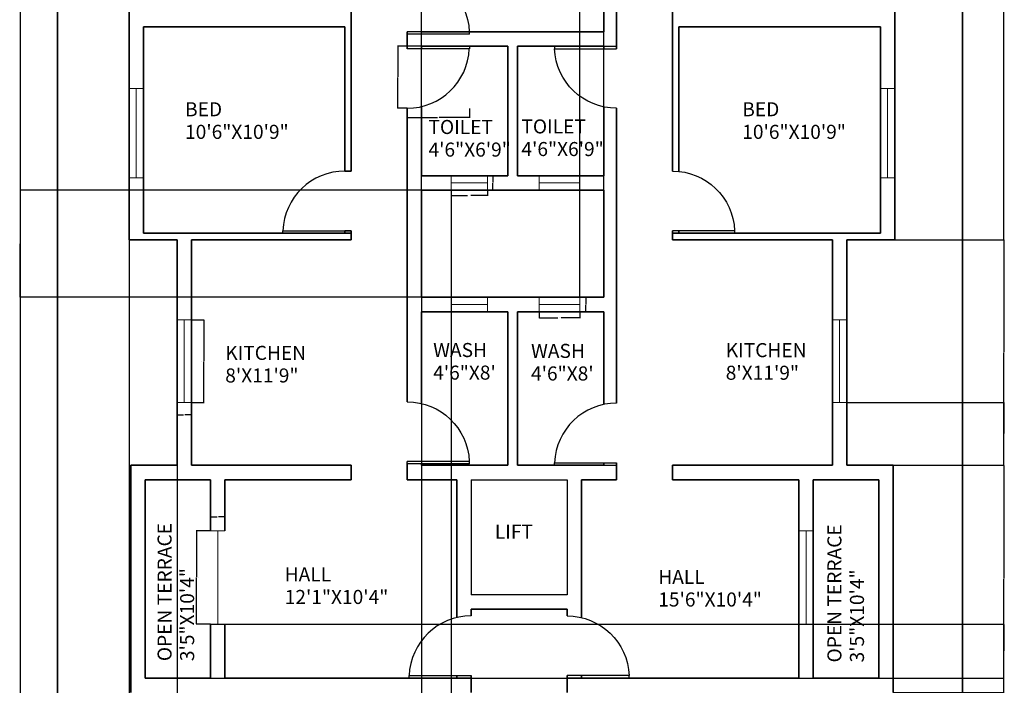
# Model space of a CAD drawing. Units: feet. Extents: x 100807 to 101423, y 154875 to 156331.
# Tile 2 of 8: x 100807 to 101423, y 155624 to 156040. Entities that reach past the tile are written whole.
import ezdxf

# ---------------------------------------------------------------- set-up
doc = ezdxf.new("R2010")
doc.units = ezdxf.units.FT
for name, color, linetype, lineweight in [('A-ANNO-DIMS', 2, 'Continuous', 18), ('A-ANNO-TTLB', 7, 'Continuous', 35), ('A-AREA-IDEN', 7, 'Continuous', 25), ('A-DOOR', 4, 'Continuous', 25), ('A-EQPM-ELEV', 8, 'Continuous', 25), ('A-GLAZ', 4, 'Continuous', 18), ('A-WALL', 7, 'Continuous', 35)]:
    doc.layers.add(name, color=color, linetype=linetype, lineweight=lineweight)
doc.styles.get("Standard").update_dxf_attribs({"font": 'arial.ttf'})
doc.dimstyles.get("Standard").update_dxf_attribs({"dimtxt": 0.18, "dimasz": 0.18, "dimexe": 0.18, "dimexo": 0.0625, "dimgap": 0.09, "dimtad": 0, "dimtih": 1, "dimtoh": 1, "dimdec": 4, "dimzin": 0, "dimdsep": 46, "dimtxsty": 'Standard', "dimcen": 0.09, "dimadec": 0, "dimazin": 0, "dimtfac": 1, "dimtdec": 4, "dimtofl": 0, "dimtmove": 0, "dimatfit": 3, "dimfxl": 1, "dimtolj": 1, "dimtzin": 0, "dimarcsym": 0})

# ---------------------------------------------------------------- blocks, each defined once
blk = doc.blocks.new('DR-36')
for p, q in [((0, 36), (0, 0)), ((0, 36), (1.5, 36)), ((1.5, 36), (1.5, 0)), ((0, 0), (1.5, 0))]:
    blk.add_line(p, q)
blk.add_arc((0, 0), 36, 0, 87.6141)
blk = doc.blocks.new('VENT-COURT-A')
for p, q in [((0, 9), (0, 0)), ((22.83, 9), (22.83, 0)), ((22.83, 4.5), (0, 4.5))]:
    blk.add_line(p, q)
blk = doc.blocks.new('VENT-COURT-B')
for p, q in [((0, 9), (0, 0)), ((25.42, 9), (25.42, 0)), ((25.42, 4.5), (0, 4.5))]:
    blk.add_line(p, q)
blk = doc.blocks.new('WIN-KITCHEN')
for p, q in [((0, 51.58), (9, 51.58)), ((4.5, 51.58), (4.5, 0)), ((0, 0), (9, 0))]:
    blk.add_line(p, q)
blk = doc.blocks.new('WIN-BED-SIDE')
for p, q in [((0, 55.85), (9, 55.85)), ((4.5, 55.85), (4.5, 0)), ((0, 0), (9, 0))]:
    blk.add_line(p, q)
blk = doc.blocks.new('WIN-TERRACE')
for p, q in [((0, 58.29), (9, 58.29)), ((4.5, 58.29), (4.5, 0)), ((0, 0), (9, 0))]:
    blk.add_line(p, q)
blk = doc.blocks.new('LIFT-OUTLINE')
for p, q in [((0, 72), (0, 0)), ((0, 72), (60, 72)), ((60, 72), (60, 0)), ((60, 72), (60, 0)), ((60, 0), (0, 0))]:
    blk.add_line(p, q)
blk = doc.blocks.new('*D12')
at = {"layer": 'A-ANNO-DIMS', "color": 0, "lineweight": -2, "transparency": 16777216}
for p, q in [((101049.09, 156023.58), (101043.15, 156023.58)), ((101043.33, 156023.4), (101043.33, 156004.33)), ((101043.33, 155984.89), (101043.33, 156003.96)), ((101049.09, 155984.71), (101043.15, 155984.71))]:
    blk.add_line(p, q, dxfattribs=at)
at = {"layer": 'A-ANNO-DIMS', "color": 0, "transparency": 16777216}
for points in [[(101043.3, 156023.4), (101043.36, 156023.4), (101043.33, 156023.58)], [(101043.3, 155984.89), (101043.36, 155984.89), (101043.33, 155984.71)]]:
    blk.add_solid(points, dxfattribs=at)
at = {"layer": 'Defpoints', "color": 0, "transparency": 16777216}
for p in [(101049.16, 156023.58), (101043.33, 155984.71), (101049.16, 155984.71)]:
    blk.add_point(p, dxfattribs=at)
at = {"layer": 'A-ANNO-DIMS', "color": 0, "transparency": 16777216, "insert": (101043.33, 156004.14), "char_height": 0.18, "attachment_point": 5}
blk.add_mtext('\\A1;DOOR 39 TYP.', dxfattribs=at)
blk = doc.blocks.new('*D13')
at = {"layer": 'A-ANNO-DIMS', "color": 0, "lineweight": -2, "transparency": 16777216}
for p, q in [((101049.16, 155984.65), (101049.16, 155978.7)), ((101088.02, 155984.65), (101088.02, 155978.7)), ((101049.34, 155978.88), (101068.06, 155978.88)), ((101087.84, 155978.88), (101069.12, 155978.88))]:
    blk.add_line(p, q, dxfattribs=at)
at = {"layer": 'A-ANNO-DIMS', "color": 0, "transparency": 16777216}
for points in [[(101049.34, 155978.91), (101049.34, 155978.85), (101049.16, 155978.88)], [(101087.84, 155978.91), (101087.84, 155978.85), (101088.02, 155978.88)]]:
    blk.add_solid(points, dxfattribs=at)
at = {"layer": 'Defpoints', "color": 0, "transparency": 16777216}
for p in [(101049.16, 155984.71), (101088.02, 155984.71), (101088.02, 155978.88)]:
    blk.add_point(p, dxfattribs=at)
at = {"layer": 'A-ANNO-DIMS', "color": 0, "transparency": 16777216, "insert": (101068.59, 155978.88), "char_height": 0.18, "attachment_point": 5}
blk.add_mtext('\\A1;39 TYP.', dxfattribs=at)
blk = doc.blocks.new('*D14')
at = {"layer": 'A-ANNO-DIMS', "color": 0, "lineweight": -2, "transparency": 16777216}
for p, q in [((101076.57, 155933.52), (101076.57, 155929.97)), ((101099.4, 155933.52), (101099.4, 155929.97)), ((101076.75, 155930.15), (101086.96, 155930.15)), ((101099.22, 155930.15), (101089, 155930.15))]:
    blk.add_line(p, q, dxfattribs=at)
at = {"layer": 'A-ANNO-DIMS', "color": 0, "transparency": 16777216}
for points in [[(101076.75, 155930.18), (101076.75, 155930.12), (101076.57, 155930.15)], [(101099.22, 155930.18), (101099.22, 155930.12), (101099.4, 155930.15)]]:
    blk.add_solid(points, dxfattribs=at)
at = {"layer": 'Defpoints', "color": 0, "transparency": 16777216}
for p in [(101076.57, 155933.58), (101099.4, 155933.58), (101099.4, 155930.15)]:
    blk.add_point(p, dxfattribs=at)
at = {"layer": 'A-ANNO-DIMS', "color": 0, "transparency": 16777216, "insert": (101087.98, 155930.15), "char_height": 0.18, "attachment_point": 5}
blk.add_mtext('\\A1;VENT A 23 TYP.', dxfattribs=at)
blk = doc.blocks.new('*D15')
at = {"layer": 'A-ANNO-DIMS', "color": 0, "lineweight": -2, "transparency": 16777216}
for p, q in [((101099.46, 155942.58), (101103, 155942.58)), ((101102.82, 155942.4), (101102.82, 155938.26)), ((101099.46, 155933.58), (101103, 155933.58)), ((101102.82, 155933.76), (101102.82, 155937.9))]:
    blk.add_line(p, q, dxfattribs=at)
at = {"layer": 'A-ANNO-DIMS', "color": 0, "transparency": 16777216}
for points in [[(101102.79, 155942.4), (101102.85, 155942.4), (101102.82, 155942.58)], [(101102.79, 155933.76), (101102.85, 155933.76), (101102.82, 155933.58)]]:
    blk.add_solid(points, dxfattribs=at)
at = {"layer": 'Defpoints', "color": 0, "transparency": 16777216}
for p in [(101099.4, 155942.58), (101102.82, 155942.58), (101099.4, 155933.58)]:
    blk.add_point(p, dxfattribs=at)
at = {"layer": 'A-ANNO-DIMS', "color": 0, "transparency": 16777216, "insert": (101102.82, 155938.08), "char_height": 0.18, "attachment_point": 5}
blk.add_mtext('\\A1;9 TYP.', dxfattribs=at)
blk = doc.blocks.new('*D16')
at = {"layer": 'A-ANNO-DIMS', "color": 0, "lineweight": -2, "transparency": 16777216}
for p, q in [((101131.66, 155857.52), (101131.66, 155853.59)), ((101131.84, 155853.77), (101143.35, 155853.77)), ((101156.9, 155853.77), (101145.39, 155853.77)), ((101157.08, 155857.52), (101157.08, 155853.59))]:
    blk.add_line(p, q, dxfattribs=at)
at = {"layer": 'A-ANNO-DIMS', "color": 0, "transparency": 16777216}
for points in [[(101131.84, 155853.8), (101131.84, 155853.74), (101131.66, 155853.77)], [(101156.9, 155853.8), (101156.9, 155853.74), (101157.08, 155853.77)]]:
    blk.add_solid(points, dxfattribs=at)
at = {"layer": 'Defpoints', "color": 0, "transparency": 16777216}
for p in [(101131.66, 155857.58), (101157.08, 155857.58), (101157.08, 155853.77)]:
    blk.add_point(p, dxfattribs=at)
at = {"layer": 'A-ANNO-DIMS', "color": 0, "transparency": 16777216, "insert": (101144.37, 155853.77), "char_height": 0.18, "attachment_point": 5}
blk.add_mtext('\\A1;VENT B 25 TYP.', dxfattribs=at)
blk = doc.blocks.new('*D17')
at = {"layer": 'A-ANNO-DIMS', "color": 0, "lineweight": -2, "transparency": 16777216}
for p, q in [((101157.14, 155866.58), (101161.07, 155866.58)), ((101160.89, 155866.4), (101160.89, 155862.26)), ((101160.89, 155857.76), (101160.89, 155861.9)), ((101157.14, 155857.58), (101161.07, 155857.58))]:
    blk.add_line(p, q, dxfattribs=at)
at = {"layer": 'A-ANNO-DIMS', "color": 0, "transparency": 16777216}
for points in [[(101160.86, 155866.4), (101160.92, 155866.4), (101160.89, 155866.58)], [(101160.86, 155857.76), (101160.92, 155857.76), (101160.89, 155857.58)]]:
    blk.add_solid(points, dxfattribs=at)
at = {"layer": 'Defpoints', "color": 0, "transparency": 16777216}
for p in [(101157.08, 155866.58), (101160.89, 155866.58), (101157.08, 155857.58)]:
    blk.add_point(p, dxfattribs=at)
at = {"layer": 'A-ANNO-DIMS', "color": 0, "transparency": 16777216, "insert": (101160.89, 155862.08), "char_height": 0.18, "attachment_point": 5}
blk.add_mtext('\\A1;9 TYP.', dxfattribs=at)
blk = doc.blocks.new('*D22')
at = {"layer": 'A-ANNO-DIMS', "color": 0, "lineweight": -2, "transparency": 16777216}
for p, q in [((100914.22, 155852.5), (100922.07, 155852.5)), ((100921.89, 155852.32), (100921.89, 155826.9)), ((100921.89, 155801.1), (100921.89, 155826.53)), ((100914.22, 155800.92), (100922.07, 155800.92))]:
    blk.add_line(p, q, dxfattribs=at)
at = {"layer": 'A-ANNO-DIMS', "color": 0, "transparency": 16777216}
for points in [[(100921.86, 155852.32), (100921.92, 155852.32), (100921.89, 155852.5)], [(100921.86, 155801.1), (100921.92, 155801.1), (100921.89, 155800.92)]]:
    blk.add_solid(points, dxfattribs=at)
at = {"layer": 'Defpoints', "color": 0, "transparency": 16777216}
for p in [(100914.16, 155852.5), (100921.89, 155852.5), (100914.16, 155800.92)]:
    blk.add_point(p, dxfattribs=at)
at = {"layer": 'A-ANNO-DIMS', "color": 0, "transparency": 16777216, "insert": (100921.89, 155826.71), "char_height": 0.18, "attachment_point": 5}
blk.add_mtext('\\A1;KITCHEN WIN. 52 TYP.', dxfattribs=at)
blk = doc.blocks.new('*D23')
at = {"layer": 'A-ANNO-DIMS', "color": 0, "lineweight": -2, "transparency": 16777216}
for p, q in [((100905.16, 155800.86), (100905.16, 155793.01)), ((100914.16, 155800.86), (100914.16, 155793.01)), ((100905.34, 155793.19), (100909.2, 155793.19)), ((100913.98, 155793.19), (100910.11, 155793.19))]:
    blk.add_line(p, q, dxfattribs=at)
at = {"layer": 'A-ANNO-DIMS', "color": 0, "transparency": 16777216}
for points in [[(100905.34, 155793.22), (100905.34, 155793.16), (100905.16, 155793.19)], [(100913.98, 155793.22), (100913.98, 155793.16), (100914.16, 155793.19)]]:
    blk.add_solid(points, dxfattribs=at)
at = {"layer": 'Defpoints', "color": 0, "transparency": 16777216}
for p in [(100905.16, 155800.92), (100914.16, 155800.92), (100914.16, 155793.19)]:
    blk.add_point(p, dxfattribs=at)
at = {"layer": 'A-ANNO-DIMS', "color": 0, "transparency": 16777216, "insert": (100909.66, 155793.19), "char_height": 0.18, "attachment_point": 5}
blk.add_mtext('\\A1;9 TYP.', dxfattribs=at)
blk = doc.blocks.new('*D26')
at = {"layer": 'A-ANNO-DIMS', "color": 0, "lineweight": -2, "transparency": 16777216}
for p, q in [((100926.09, 155720.64), (100917.23, 155720.64)), ((100917.41, 155720.46), (100917.41, 155691.68)), ((100917.41, 155662.53), (100917.41, 155691.31)), ((100926.09, 155662.35), (100917.23, 155662.35))]:
    blk.add_line(p, q, dxfattribs=at)
at = {"layer": 'A-ANNO-DIMS', "color": 0, "transparency": 16777216}
for points in [[(100917.38, 155720.46), (100917.44, 155720.46), (100917.41, 155720.64)], [(100917.38, 155662.53), (100917.44, 155662.53), (100917.41, 155662.35)]]:
    blk.add_solid(points, dxfattribs=at)
at = {"layer": 'Defpoints', "color": 0, "transparency": 16777216}
for p in [(100917.41, 155720.64), (100926.16, 155720.64), (100926.16, 155662.35)]:
    blk.add_point(p, dxfattribs=at)
at = {"layer": 'A-ANNO-DIMS', "color": 0, "transparency": 16777216, "insert": (100917.41, 155691.5), "char_height": 0.18, "attachment_point": 5}
blk.add_mtext('\\A1;TERRACE WIN. 58 TYP.', dxfattribs=at)
blk = doc.blocks.new('*D27')
at = {"layer": 'A-ANNO-DIMS', "color": 0, "lineweight": -2, "transparency": 16777216}
for p, q in [((100926.16, 155720.7), (100926.16, 155729.57)), ((100926.34, 155729.39), (100930.2, 155729.39)), ((100934.98, 155729.39), (100931.11, 155729.39)), ((100935.16, 155720.7), (100935.16, 155729.57))]:
    blk.add_line(p, q, dxfattribs=at)
at = {"layer": 'A-ANNO-DIMS', "color": 0, "transparency": 16777216}
for points in [[(100926.34, 155729.42), (100926.34, 155729.36), (100926.16, 155729.39)], [(100934.98, 155729.42), (100934.98, 155729.36), (100935.16, 155729.39)]]:
    blk.add_solid(points, dxfattribs=at)
at = {"layer": 'Defpoints', "color": 0, "transparency": 16777216}
for p in [(100935.16, 155729.39), (100926.16, 155720.64), (100935.16, 155720.64)]:
    blk.add_point(p, dxfattribs=at)
at = {"layer": 'A-ANNO-DIMS', "color": 0, "transparency": 16777216, "insert": (100930.66, 155729.39), "char_height": 0.18, "attachment_point": 5}
blk.add_mtext('\\A1;9 TYP.', dxfattribs=at)
blk = doc.blocks.new('*D35')
at = {"layer": 'A-ANNO-DIMS', "color": 0, "lineweight": -2, "transparency": 16777216}
for p, q in [((100875.09, 156234.58), (100806.83, 156234.58)), ((100807.01, 156234.4), (100807.01, 155589.76)), ((100807.01, 154944.76), (100807.01, 155589.4)), ((100875.09, 154944.58), (100806.83, 154944.58))]:
    blk.add_line(p, q, dxfattribs=at)
at = {"layer": 'A-ANNO-DIMS', "color": 0, "transparency": 16777216}
for points in [[(100806.98, 156234.4), (100807.04, 156234.4), (100807.01, 156234.58)], [(100806.98, 154944.76), (100807.04, 154944.76), (100807.01, 154944.58)]]:
    blk.add_solid(points, dxfattribs=at)
at = {"layer": 'Defpoints', "color": 0, "transparency": 16777216}
for p in [(100807.01, 156234.58), (100875.16, 156234.58), (100875.16, 154944.58)]:
    blk.add_point(p, dxfattribs=at)
at = {"layer": 'A-ANNO-DIMS', "color": 0, "transparency": 16777216, "insert": (100807.01, 155589.58), "char_height": 0.18, "attachment_point": 5}
blk.add_mtext('\\A1;1290', dxfattribs=at)
blk = doc.blocks.new('*D36')
at = {"layer": 'A-ANNO-DIMS', "color": 0, "lineweight": -2, "transparency": 16777216}
for p, q in [((101058.16, 155866.64), (101058.16, 156302.91)), ((101172.16, 155866.64), (101172.16, 156302.91)), ((101058.34, 156302.73), (101114.88, 156302.73)), ((101171.98, 156302.73), (101115.44, 156302.73))]:
    blk.add_line(p, q, dxfattribs=at)
at = {"layer": 'A-ANNO-DIMS', "color": 0, "transparency": 16777216}
for points in [[(101058.34, 156302.76), (101058.34, 156302.7), (101058.16, 156302.73)], [(101171.98, 156302.76), (101171.98, 156302.7), (101172.16, 156302.73)]]:
    blk.add_solid(points, dxfattribs=at)
at = {"layer": 'Defpoints', "color": 0, "transparency": 16777216}
for p in [(101172.16, 156302.73), (101058.16, 155866.58), (101172.16, 155866.58)]:
    blk.add_point(p, dxfattribs=at)
at = {"layer": 'A-ANNO-DIMS', "color": 0, "transparency": 16777216, "insert": (101115.16, 156302.73), "char_height": 0.18, "attachment_point": 5}
blk.add_mtext('\\A1;114', dxfattribs=at)
blk = doc.blocks.new('*D37')
at = {"layer": 'A-ANNO-DIMS', "color": 0, "lineweight": -2, "transparency": 16777216}
for p, q in [((101058.09, 155933.58), (100806.83, 155933.58)), ((100807.01, 155933.4), (100807.01, 155900.26)), ((100807.01, 155866.76), (100807.01, 155899.9)), ((101058.09, 155866.58), (100806.83, 155866.58))]:
    blk.add_line(p, q, dxfattribs=at)
at = {"layer": 'A-ANNO-DIMS', "color": 0, "transparency": 16777216}
for points in [[(100806.98, 155933.4), (100807.04, 155933.4), (100807.01, 155933.58)], [(100806.98, 155866.76), (100807.04, 155866.76), (100807.01, 155866.58)]]:
    blk.add_solid(points, dxfattribs=at)
at = {"layer": 'Defpoints', "color": 0, "transparency": 16777216}
for p in [(100807.01, 155933.58), (101058.16, 155933.58), (101058.16, 155866.58)]:
    blk.add_point(p, dxfattribs=at)
at = {"layer": 'A-ANNO-DIMS', "color": 0, "transparency": 16777216, "insert": (100807.01, 155900.08), "char_height": 0.18, "attachment_point": 5}
blk.add_mtext('\\A1;67', dxfattribs=at)
blk = doc.blocks.new('*D41')
at = {"layer": 'A-ANNO-DIMS', "color": 0, "lineweight": -2, "transparency": 16777216}
for p, q in [((101354.22, 156234.58), (101422.49, 156234.58)), ((101422.31, 156234.4), (101422.31, 156068.76)), ((101422.31, 155902.76), (101422.31, 156068.4)), ((101354.22, 155902.58), (101422.49, 155902.58))]:
    blk.add_line(p, q, dxfattribs=at)
at = {"layer": 'A-ANNO-DIMS', "color": 0, "transparency": 16777216}
for points in [[(101422.28, 156234.4), (101422.34, 156234.4), (101422.31, 156234.58)], [(101422.28, 155902.76), (101422.34, 155902.76), (101422.31, 155902.58)]]:
    blk.add_solid(points, dxfattribs=at)
at = {"layer": 'Defpoints', "color": 0, "transparency": 16777216}
for p in [(101354.16, 156234.58), (101422.31, 156234.58), (101354.16, 155902.58)]:
    blk.add_point(p, dxfattribs=at)
at = {"layer": 'A-ANNO-DIMS', "color": 0, "transparency": 16777216, "insert": (101422.31, 156068.58), "char_height": 0.18, "attachment_point": 5}
blk.add_mtext('\\A1;332', dxfattribs=at)
blk = doc.blocks.new('*D42')
at = {"layer": 'A-ANNO-DIMS', "color": 0, "lineweight": -2, "transparency": 16777216}
for p, q in [((101354.22, 155902.58), (101422.49, 155902.58)), ((101422.31, 155902.4), (101422.31, 155832.26)), ((101422.31, 155761.76), (101422.31, 155831.9)), ((101353.22, 155761.58), (101422.49, 155761.58))]:
    blk.add_line(p, q, dxfattribs=at)
at = {"layer": 'A-ANNO-DIMS', "color": 0, "transparency": 16777216}
for points in [[(101422.28, 155902.4), (101422.34, 155902.4), (101422.31, 155902.58)], [(101422.28, 155761.76), (101422.34, 155761.76), (101422.31, 155761.58)]]:
    blk.add_solid(points, dxfattribs=at)
at = {"layer": 'Defpoints', "color": 0, "transparency": 16777216}
for p in [(101354.16, 155902.58), (101422.31, 155902.58), (101353.16, 155761.58)]:
    blk.add_point(p, dxfattribs=at)
at = {"layer": 'A-ANNO-DIMS', "color": 0, "transparency": 16777216, "insert": (101422.31, 155832.08), "char_height": 0.18, "attachment_point": 5}
blk.add_mtext('\\A1;141', dxfattribs=at)
blk = doc.blocks.new('*D43')
at = {"layer": 'A-ANNO-DIMS', "color": 0, "lineweight": -2, "transparency": 16777216}
for p, q in [((101353.22, 155761.58), (101422.49, 155761.58)), ((101422.31, 155761.4), (101422.31, 155690.75)), ((101422.31, 155619.74), (101422.31, 155690.38)), ((101353.22, 155619.56), (101422.49, 155619.56))]:
    blk.add_line(p, q, dxfattribs=at)
at = {"layer": 'A-ANNO-DIMS', "color": 0, "transparency": 16777216}
for points in [[(101422.28, 155761.4), (101422.34, 155761.4), (101422.31, 155761.58)], [(101422.28, 155619.74), (101422.34, 155619.74), (101422.31, 155619.56)]]:
    blk.add_solid(points, dxfattribs=at)
at = {"layer": 'Defpoints', "color": 0, "transparency": 16777216}
for p in [(101353.16, 155761.58), (101422.31, 155761.58), (101353.16, 155619.56)]:
    blk.add_point(p, dxfattribs=at)
at = {"layer": 'A-ANNO-DIMS', "color": 0, "transparency": 16777216, "insert": (101422.31, 155690.57), "char_height": 0.18, "attachment_point": 5}
blk.add_mtext('\\A1;142.02', dxfattribs=at)
blk = doc.blocks.new('*D45')
at = {"layer": 'A-ANNO-DIMS', "color": 0, "lineweight": -2, "transparency": 16777216}
for p, q in [((100875.16, 155902.52), (100875.16, 154876.25)), ((100905.16, 155902.52), (100905.16, 154876.25)), ((100875.34, 154876.43), (100889.94, 154876.43)), ((100904.98, 154876.43), (100890.37, 154876.43))]:
    blk.add_line(p, q, dxfattribs=at)
at = {"layer": 'A-ANNO-DIMS', "color": 0, "transparency": 16777216}
for points in [[(100875.34, 154876.46), (100875.34, 154876.4), (100875.16, 154876.43)], [(100904.98, 154876.46), (100904.98, 154876.4), (100905.16, 154876.43)]]:
    blk.add_solid(points, dxfattribs=at)
at = {"layer": 'Defpoints', "color": 0, "transparency": 16777216}
for p in [(100875.16, 155902.58), (100905.16, 155902.58), (100905.16, 154876.43)]:
    blk.add_point(p, dxfattribs=at)
at = {"layer": 'A-ANNO-DIMS', "color": 0, "transparency": 16777216, "insert": (100890.16, 154876.43), "char_height": 0.18, "attachment_point": 5}
blk.add_mtext('\\A1;30', dxfattribs=at)
blk = doc.blocks.new('*D48')
at = {"layer": 'A-ANNO-DIMS', "color": 0, "lineweight": -2, "transparency": 16777216}
for p, q in [((101058.16, 155933.52), (101058.16, 154876.25)), ((101076.57, 155933.52), (101076.57, 154876.25)), ((101058.34, 154876.43), (101066.99, 154876.43)), ((101076.39, 154876.43), (101067.73, 154876.43))]:
    blk.add_line(p, q, dxfattribs=at)
at = {"layer": 'A-ANNO-DIMS', "color": 0, "transparency": 16777216}
for points in [[(101058.34, 154876.46), (101058.34, 154876.4), (101058.16, 154876.43)], [(101076.39, 154876.46), (101076.39, 154876.4), (101076.57, 154876.43)]]:
    blk.add_solid(points, dxfattribs=at)
at = {"layer": 'Defpoints', "color": 0, "transparency": 16777216}
for p in [(101058.16, 155933.58), (101076.57, 155933.58), (101076.57, 154876.43)]:
    blk.add_point(p, dxfattribs=at)
at = {"layer": 'A-ANNO-DIMS', "color": 0, "transparency": 16777216, "insert": (101067.36, 154876.43), "char_height": 0.18, "attachment_point": 5}
blk.add_mtext('\\A1;18.41', dxfattribs=at)
blk = doc.blocks.new('*D49')
at = {"layer": 'A-ANNO-DIMS', "color": 0, "lineweight": -2, "transparency": 16777216}
for p, q in [((101157.08, 155866.64), (101157.08, 156302.91)), ((101172.16, 155866.64), (101172.16, 156302.91)), ((101157.26, 156302.73), (101164.16, 156302.73)), ((101171.98, 156302.73), (101165.07, 156302.73))]:
    blk.add_line(p, q, dxfattribs=at)
at = {"layer": 'A-ANNO-DIMS', "color": 0, "transparency": 16777216}
for points in [[(101157.26, 156302.76), (101157.26, 156302.7), (101157.08, 156302.73)], [(101171.98, 156302.76), (101171.98, 156302.7), (101172.16, 156302.73)]]:
    blk.add_solid(points, dxfattribs=at)
at = {"layer": 'Defpoints', "color": 0, "transparency": 16777216}
for p in [(101172.16, 156302.73), (101157.08, 155866.58), (101172.16, 155866.58)]:
    blk.add_point(p, dxfattribs=at)
at = {"layer": 'A-ANNO-DIMS', "color": 0, "transparency": 16777216, "insert": (101164.62, 156302.73), "char_height": 0.18, "attachment_point": 5}
blk.add_mtext('\\A1;15.075', dxfattribs=at)
blk = doc.blocks.new('*D51')
at = {"layer": 'A-ANNO-DIMS', "color": 0, "lineweight": -2, "transparency": 16777216}
for p, q in [((101324.22, 155800.92), (101422.49, 155800.92)), ((101422.31, 155800.74), (101422.31, 155781.43)), ((101422.31, 155761.76), (101422.31, 155781.07)), ((101324.22, 155761.58), (101422.49, 155761.58))]:
    blk.add_line(p, q, dxfattribs=at)
at = {"layer": 'A-ANNO-DIMS', "color": 0, "transparency": 16777216}
for points in [[(101422.28, 155800.74), (101422.34, 155800.74), (101422.31, 155800.92)], [(101422.28, 155761.76), (101422.34, 155761.76), (101422.31, 155761.58)]]:
    blk.add_solid(points, dxfattribs=at)
at = {"layer": 'Defpoints', "color": 0, "transparency": 16777216}
for p in [(101324.16, 155800.92), (101422.31, 155800.92), (101324.16, 155761.58)]:
    blk.add_point(p, dxfattribs=at)
at = {"layer": 'A-ANNO-DIMS', "color": 0, "transparency": 16777216, "insert": (101422.31, 155781.25), "char_height": 0.18, "attachment_point": 5}
blk.add_mtext('\\A1;39.35', dxfattribs=at)
blk = doc.blocks.new('*D53')
at = {"layer": 'A-ANNO-DIMS', "color": 0, "lineweight": -2, "transparency": 16777216}
for p, q in [((100926.22, 155662.35), (101422.49, 155662.35)), ((101422.31, 155662.17), (101422.31, 155645.65)), ((101422.31, 155628.76), (101422.31, 155645.28)), ((100926.22, 155628.58), (101422.49, 155628.58))]:
    blk.add_line(p, q, dxfattribs=at)
at = {"layer": 'A-ANNO-DIMS', "color": 0, "transparency": 16777216}
for points in [[(101422.28, 155662.17), (101422.34, 155662.17), (101422.31, 155662.35)], [(101422.28, 155628.76), (101422.34, 155628.76), (101422.31, 155628.58)]]:
    blk.add_solid(points, dxfattribs=at)
at = {"layer": 'Defpoints', "color": 0, "transparency": 16777216}
for p in [(100926.16, 155662.35), (101422.31, 155662.35), (100926.16, 155628.58)]:
    blk.add_point(p, dxfattribs=at)
at = {"layer": 'A-ANNO-DIMS', "color": 0, "transparency": 16777216, "insert": (101422.31, 155645.47), "char_height": 0.18, "attachment_point": 5}
blk.add_mtext('\\A1;33.776', dxfattribs=at)

msp = doc.modelspace()

# ---------------------------------------------------------------- linework, layer by layer
at = {"layer": 'A-ANNO-TTLB'}
msp.add_lwpolyline([(100830.3877, 156331.4447), (101396.4426, 156331.4447), (101396.4426, 154875.4601), (100830.3877, 154875.4601)], close=True, dxfattribs=at)
at = {"layer": 'A-WALL'}
for p, q in [((100875.1564, 156035.5777), (100875.1564, 156234.5777)), ((101354.1564, 156035.5777), (101354.1564, 156234.5777)), ((101172.1564, 156156.5789), (101172.1564, 156032.5789)), ((101014.1564, 155945.4274), (101014.1564, 156101.5777)), ((101180.1564, 156092.5777), (101180.1564, 156021.9594)), ((101215.1564, 155945.4459), (101215.1564, 156092.5777)), ((100875.1564, 156035.5777), (100875.1564, 155902.5777)), ((101010.1564, 156035.5777), (100884.1564, 156035.5777)), ((100884.1564, 156035.5777), (100884.1564, 155906.5777)), ((101010.1564, 155945.4459), (101010.1564, 156035.5777)), ((101049.1564, 156032.5789), (101049.1564, 156021.9594)), ((101172.1564, 156032.5789), (101058.1564, 156032.5789)), ((101219.1564, 156035.5777), (101345.1564, 156035.5777)), ((101219.1564, 155945.2396), (101219.1564, 156035.5777)), ((101345.1564, 156035.5777), (101345.1564, 155906.5777)), ((101354.1564, 156035.5777), (101354.1564, 155902.5777)), ((101112.1564, 156023.5789), (101058.1564, 156023.5789)), ((101058.1564, 156023.5789), (101058.1564, 156021.9594)), ((101112.1564, 156023.5789), (101112.1564, 155942.5789)), ((101172.1564, 156023.5789), (101118.1564, 156023.5789)), ((101118.1564, 156023.5789), (101118.1564, 155942.5789)), ((101172.1564, 156023.5789), (101172.1564, 156021.9594)), ((101049.1564, 155984.7107), (101049.1564, 155801.2566)), ((101058.1564, 155985.7671), (101058.1564, 155942.5789)), ((101172.1564, 155985.5429), (101172.1564, 155942.5789)), ((101180.1564, 155984.7107), (101180.1564, 155800.4459)), ((101010.1564, 155945.4459), (101014.1564, 155945.4274)), ((101112.1564, 155942.5789), (101058.1564, 155942.5789)), ((101172.1564, 155942.5789), (101118.1564, 155942.5789)), ((101172.1564, 155933.5789), (101058.1564, 155933.5789)), ((101058.1564, 155933.5789), (101058.1564, 155866.5789)), ((101172.1564, 155933.5789), (101118.1564, 155933.5789)), ((101172.1564, 155933.5789), (101172.1564, 155866.5789)), ((100905.1564, 155902.5777), (100875.1564, 155902.5777)), ((100884.1564, 155906.5777), (101014.1564, 155906.5777)), ((100905.1564, 155902.5777), (100905.1564, 155761.5777)), ((100914.1564, 155902.5777), (101010.1564, 155902.5777)), ((100914.1564, 155902.5777), (100914.1564, 155761.5777)), ((101010.1564, 155906.5777), (101010.1564, 155908.1972)), ((101010.1564, 155908.1972), (101014.1564, 155908.1972)), ((101010.1564, 155902.5777), (101014.1564, 155902.5777)), ((101014.1564, 155902.5777), (101014.1564, 155908.1972)), ((101215.1564, 155902.5777), (101215.1564, 155908.1972)), ((101345.1564, 155906.5777), (101215.1564, 155906.5777)), ((101219.1564, 155902.5777), (101215.1564, 155902.5777)), ((101219.1564, 155906.5777), (101219.1564, 155908.1972)), ((101315.1564, 155902.5777), (101219.1564, 155902.5777)), ((101315.1564, 155902.5777), (101315.1564, 155761.5777)), ((101324.1564, 155902.5777), (101324.1564, 155761.5777)), ((101324.1564, 155902.5777), (101354.1564, 155902.5777)), ((101058.1564, 155866.5789), (101172.1564, 155866.5789)), ((101058.1564, 155857.5789), (101112.1564, 155857.5789)), ((101058.1564, 155857.5789), (101058.1564, 155800.2002)), ((101112.1564, 155857.5789), (101112.1564, 155761.5777)), ((101118.1564, 155857.5789), (101118.1564, 155761.5777)), ((101118.1564, 155857.5789), (101172.1564, 155857.5789)), ((101172.1564, 155857.5789), (101172.1564, 155799.6137)), ((100905.1564, 155761.5777), (100876.1564, 155761.5777)), ((100876.1564, 155761.5777), (100876.1564, 155619.5777)), ((100914.1564, 155761.5777), (101010.1564, 155761.5777)), ((100935.1564, 155761.5777), (101014.1564, 155761.5777)), ((101014.1564, 155761.5777), (101014.1564, 155752.5777)), ((101049.1564, 155763.199), (101049.1564, 155761.5777)), ((101049.1564, 155761.5777), (101049.1564, 155752.5777)), ((101058.1564, 155762.3883), (101058.1564, 155761.5789)), ((101112.1564, 155761.5777), (101058.1564, 155761.5789)), ((101118.1564, 155761.5777), (101161.1564, 155761.5777)), ((101161.1564, 155761.5777), (101172.1564, 155761.5777)), ((101172.1564, 155763.1972), (101172.1564, 155761.5777)), ((101180.1564, 155763.1972), (101180.1564, 155761.5777)), ((101180.1564, 155761.5777), (101180.1564, 155752.5777)), ((101294.1564, 155761.5777), (101215.1564, 155761.5777)), ((101215.1564, 155761.5777), (101215.1564, 155752.5777)), ((101315.1564, 155761.5777), (101219.1564, 155761.5777)), ((101324.1564, 155761.5777), (101353.1564, 155761.5777)), ((101353.1564, 155761.5777), (101353.1564, 155619.5557)), ((100914.1564, 155752.5777), (100885.1564, 155752.5777)), ((100885.1564, 155752.5777), (100885.1564, 155628.5777)), ((100914.1564, 155752.5777), (100926.1564, 155752.5777)), ((100926.1564, 155720.6421), (100926.1564, 155752.5777)), ((100935.1564, 155752.5777), (101014.1564, 155752.5777)), ((100935.1564, 155720.6421), (100935.1564, 155752.5777)), ((101049.1564, 155752.5777), (101080.1564, 155752.5777)), ((101080.1564, 155752.5777), (101080.1564, 155666.3896)), ((101158.1564, 155752.5777), (101158.1564, 155666.3896)), ((101158.1564, 155752.5777), (101180.1564, 155752.5777)), ((101180.1564, 155752.5777), (101158.1564, 155752.5777)), ((101294.1564, 155752.5777), (101215.1564, 155752.5777)), ((101294.1564, 155628.5777), (101294.1564, 155752.5777)), ((101315.1564, 155752.5777), (101303.1564, 155752.5777)), ((101303.1564, 155628.5777), (101303.1564, 155752.5777)), ((101315.1564, 155752.5777), (101344.1564, 155752.5777)), ((101344.1564, 155752.5777), (101344.1564, 155628.5777)), ((101149.1564, 155671.5777), (101089.1564, 155671.5777)), ((101089.1564, 155671.5777), (101089.1564, 155667.4459)), ((101149.1564, 155671.5777), (101149.1564, 155667.4459)), ((100926.1564, 155628.5777), (100926.1564, 155662.354)), ((100935.1564, 155628.5777), (100935.1564, 155662.354)), ((100885.1564, 155628.5777), (100926.1564, 155628.5777)), ((101080.1564, 155628.5777), (100935.1564, 155628.5777)), ((101080.1564, 155630.1972), (101080.1564, 155628.5777)), ((101080.1564, 155628.5777), (101089.1564, 155628.5777)), ((101089.1564, 155630.1972), (101089.1564, 155619.5777)), ((101149.1564, 155630.1972), (101149.1564, 155628.5777)), ((101149.1564, 155628.5777), (101294.1564, 155628.5777)), ((101149.1564, 155628.5777), (101149.1564, 155619.5777)), ((101158.1564, 155630.1972), (101158.1564, 155628.5777)), ((101344.1564, 155628.5777), (101303.1564, 155628.5777))]:
    msp.add_line(p, q, dxfattribs=at)

# ---------------------------------------------------------------- block references
at = {"layer": 'A-DOOR', "yscale": 1.079672442471032, "zscale": 1.079672442471032}
for p, xscale, rotation in [((101049.1564, 156030.9594), -1.079672442471032, 270.0000000000369), ((101049.1564, 156023.5789), 1.079672442471032, 269.9999999999631), ((101180.1564, 156023.5789), -1.079672442471032, 90), ((101010.1564, 155906.5777), 1.079672442471032, 90), ((101215.1564, 155906.5777), -1.079672442471032, 270.0000000000369), ((101049.1564, 155762.3883), -1.079672442471032, 270.0000000000369), ((101180.1564, 155761.5777), 1.079672442471032, 90), ((101089.1564, 155628.5777), 1.079672442471032, 90), ((101149.1564, 155628.5777), -1.079672442471032, 270.0000000000369)]:
    msp.add_blockref('DR-36', p, dxfattribs=dict(at, xscale=xscale, rotation=rotation))
at = {"layer": 'A-EQPM-ELEV'}
msp.add_blockref('LIFT-OUTLINE', (101089.1564, 155680.5777), dxfattribs=at)
at = {"layer": 'A-GLAZ'}
for name, p in [('WIN-BED-SIDE', (100875.1564, 155941.303)), ('VENT-COURT-A', (101076.5662, 155933.5789)), ('VENT-COURT-B', (101131.6622, 155933.5789)), ('VENT-COURT-B', (101131.6622, 155857.5789)), ('WIN-KITCHEN', (100905.1564, 155800.9242)), ('WIN-KITCHEN', (101315.1564, 155800.9242)), ('WIN-TERRACE', (100926.1564, 155662.354))]:
    msp.add_blockref(name, p, dxfattribs=at)
at = {"layer": 'A-GLAZ', "rotation": 180}
for name, p in [('WIN-BED-SIDE', (101354.1564, 155997.1501)), ('VENT-COURT-A', (101099.3962, 155866.5789)), ('WIN-TERRACE', (101303.1564, 155720.6421))]:
    msp.add_blockref(name, p, dxfattribs=at)

# ---------------------------------------------------------------- texts
at = {"layer": 'A-ANNO-DIMS'}
for s, height, p in [('10\'6"X10\'9"', 8.788223, (100910.1724, 155965.5882)), ('10\'6"X10\'9"', 8.788223, (101258.7501, 155965.5882)), ('4\'6"X6\'9"', 8.78822, (101120.5911, 155954.8526)), ('4\'6"X6\'9"', 8.78822, (101062.4577, 155954.5148)), ('8\'X11\'9"', 8.78822, (100935.3222, 155813.3282)), ('4\'6"X8\'', 8.78822, (101065.3908, 155815.1121)), ('4\'6"X8\'', 8.78822, (101126.6018, 155814.5708)), ('8\'X11\'9"', 8.78822, (101248.4226, 155815.0284)), ('12\'1"X10\'4"', 8.788223, (100972.5123, 155674.879)), ('15\'6"X10\'4"', 8.788223, (101206.2046, 155673.3007))]:
    msp.add_text(s, height=height, dxfattribs=at).set_placement(p)
for p in [(100915.8734, 155639.1626), (101334.9102, 155638.345)]:
    msp.add_text('3\'5"X10\'4"', height=8.78822, rotation=90, dxfattribs=at).set_placement(p)
at = {"layer": 'A-AREA-IDEN'}
for s, p in [('BED', (100910.1724, 155979.7057)), ('BED', (101258.7501, 155979.7057)), ('TOILET', (101062.4577, 155968.6323)), ('TOILET', (101120.5911, 155968.9701)), ('KITCHEN', (100935.3222, 155827.4457)), ('WASH', (101065.3908, 155829.2296)), ('WASH', (101126.6018, 155828.6883)), ('KITCHEN', (101248.4226, 155829.1459)), ('LIFT', (101103.949, 155715.7026)), ('HALL', (100972.5123, 155688.9965)), ('HALL', (101206.2046, 155687.4182))]:
    msp.add_text(s, height=8.78822, dxfattribs=at).set_placement(p)
for p in [(100901.7559, 155639.1626), (101320.7927, 155638.345)]:
    msp.add_text('OPEN TERRACE', height=8.788223, rotation=90, dxfattribs=at).set_placement(p)

# ---------------------------------------------------------------- dimensions: what is measured, and where the dimension line sits
at = {"layer": 'A-ANNO-DIMS'}
for base, p1, p2, override, picture, middle in [((101172.1564, 156302.7277), (101058.1564, 155866.5789), (101172.1564, 155866.5789), {"dimdec": 0, "dimlfac": 1, "dimrnd": 0, "dimzin": 0, "dimdsep": 46, "dimlunit": 2}, '*D36', (101115.1564, 156302.7277)), ((101172.1564, 156302.7277), (101157.0816, 155866.5789), (101172.1564, 155866.5789), {"dimdec": 3, "dimlfac": 1, "dimrnd": 0, "dimzin": 0, "dimdsep": 46, "dimlunit": 2}, '*D49', (101164.619, 156302.7277)), ((101076.5662, 154876.4277), (101058.1564, 155933.5789), (101076.5662, 155933.5789), {"dimdec": 2, "dimlfac": 1, "dimrnd": 0, "dimzin": 0, "dimdsep": 46, "dimlunit": 2}, '*D48', (101067.3613, 154876.4277)), ((100905.1564, 154876.4277), (100875.1564, 155902.5777), (100905.1564, 155902.5777), {"dimdec": 0, "dimlfac": 1, "dimrnd": 0, "dimzin": 0, "dimdsep": 46, "dimlunit": 2}, '*D45', (100890.1564, 154876.4277))]:
    dim = msp.add_linear_dim(base=base, p1=p1, p2=p2, dimstyle='Standard', override=override, dxfattribs=at)
    dim.commit()
    dim.dimension.update_dxf_attribs({"geometry": picture, "text_midpoint": middle})
for base, p1, p2, override, picture, middle in [((100807.0064, 156234.5777), (100875.1564, 154944.5777), (100875.1564, 156234.5777), {"dimdec": 0, "dimlfac": 1, "dimrnd": 0, "dimzin": 0, "dimdsep": 46, "dimlunit": 2}, '*D35', (100807.0064, 155589.5777)), ((101422.3064, 156234.5777), (101354.1564, 155902.5777), (101354.1564, 156234.5777), {"dimdec": 0, "dimlfac": 1, "dimrnd": 0, "dimzin": 0, "dimdsep": 46, "dimlunit": 2}, '*D41', (101422.3064, 156068.5777)), ((100807.0064, 155933.5789), (101058.1564, 155866.5789), (101058.1564, 155933.5789), {"dimdec": 0, "dimlfac": 1, "dimrnd": 0, "dimzin": 0, "dimdsep": 46, "dimlunit": 2}, '*D37', (100807.0064, 155900.0789)), ((101422.3064, 155902.5777), (101353.1564, 155761.5777), (101354.1564, 155902.5777), {"dimdec": 0, "dimlfac": 1, "dimrnd": 0, "dimzin": 0, "dimdsep": 46, "dimlunit": 2}, '*D42', (101422.3064, 155832.0777)), ((101422.3064, 155800.9242), (101324.1564, 155761.5777), (101324.1564, 155800.9242), {"dimdec": 2, "dimlfac": 1, "dimrnd": 0, "dimzin": 0, "dimdsep": 46, "dimlunit": 2}, '*D51', (101422.3064, 155781.251)), ((101422.3064, 155761.5777), (101353.1564, 155619.5557), (101353.1564, 155761.5777), {"dimdec": 2, "dimlfac": 1, "dimrnd": 0, "dimzin": 0, "dimdsep": 46, "dimlunit": 2}, '*D43', (101422.3064, 155690.5667)), ((101422.3064, 155662.354), (100926.1564, 155628.5777), (100926.1564, 155662.354), {"dimdec": 3, "dimlfac": 1, "dimrnd": 0, "dimzin": 0, "dimdsep": 46, "dimlunit": 2}, '*D53', (101422.3064, 155645.4659))]:
    dim = msp.add_linear_dim(base=base, p1=p1, p2=p2, angle=90, dimstyle='Standard', override=override, dxfattribs=at)
    dim.commit()
    dim.dimension.update_dxf_attribs({"geometry": picture, "text_midpoint": middle})
for base, p1, p2, angle, text, picture, middle in [((101043.3262, 155984.7107), (101049.1564, 156023.5789), (101049.1564, 155984.7107), 270, 'DOOR <> TYP.', '*D12', (101043.3262, 156004.1448)), ((101102.8207, 155942.5789), (101099.3962, 155933.5789), (101099.3962, 155942.5789), 90, '<> TYP.', '*D15', (101102.8207, 155938.0789)), ((101160.8945, 155866.5789), (101157.0816, 155857.5789), (101157.0816, 155866.5789), 90, '<> TYP.', '*D17', (101160.8945, 155862.0789)), ((100921.8933, 155852.5036), (100914.1564, 155800.9242), (100914.1564, 155852.5036), 90, 'KITCHEN WIN. <> TYP.', '*D22', (100921.8933, 155826.7139)), ((100917.4132, 155720.6421), (100926.1564, 155662.354), (100926.1564, 155720.6421), 90, 'TERRACE WIN. <> TYP.', '*D26', (100917.4132, 155691.498))]:
    dim = msp.add_linear_dim(base=base, p1=p1, p2=p2, angle=angle, text=text, dimstyle='Standard', override={"dimdec": 0, "dimlfac": 1, "dimrnd": 0, "dimzin": 0, "dimdsep": 46, "dimlunit": 2}, dxfattribs=at)
    dim.commit()
    dim.dimension.update_dxf_attribs({"geometry": picture, "text_midpoint": middle})
for base, p1, p2, text, picture, middle in [((101088.0246, 155978.8805), (101049.1564, 155984.7107), (101088.0246, 155984.7107), '<> TYP.', '*D13', (101068.5905, 155978.8805)), ((101099.3962, 155930.1544), (101076.5662, 155933.5789), (101099.3962, 155933.5789), 'VENT A <> TYP.', '*D14', (101087.9812, 155930.1544)), ((101157.0816, 155853.766), (101131.6622, 155857.5789), (101157.0816, 155857.5789), 'VENT B <> TYP.', '*D16', (101144.3719, 155853.766)), ((100914.1564, 155793.1873), (100905.1564, 155800.9242), (100914.1564, 155800.9242), '<> TYP.', '*D23', (100909.6564, 155793.1873)), ((100935.1564, 155729.3853), (100926.1564, 155720.6421), (100935.1564, 155720.6421), '<> TYP.', '*D27', (100930.6564, 155729.3853))]:
    dim = msp.add_linear_dim(base=base, p1=p1, p2=p2, text=text, dimstyle='Standard', override={"dimdec": 0, "dimlfac": 1, "dimrnd": 0, "dimzin": 0, "dimdsep": 46, "dimlunit": 2}, dxfattribs=at)
    dim.commit()
    dim.dimension.update_dxf_attribs({"geometry": picture, "text_midpoint": middle})

doc.saveas('drawing.dxf')
